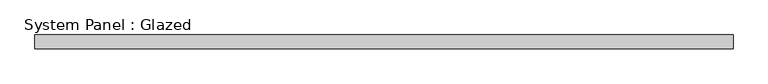
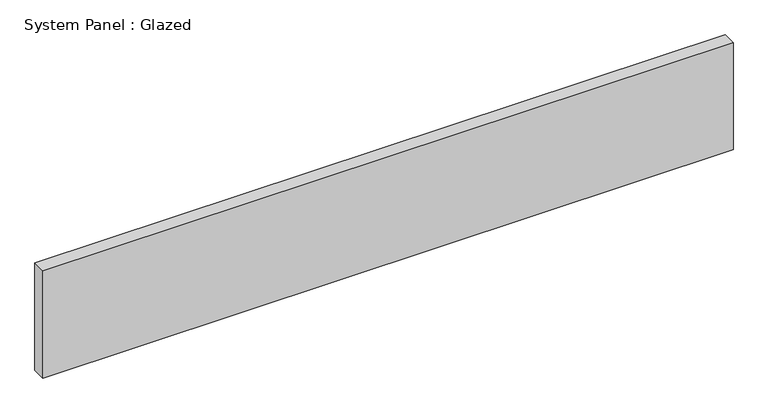
"""IFC4 building model written with IfcOpenShell, lengths in millimetres: plate geometry, System Panel : Glazed."""

from ifc_helpers import new_model, si_unit, origin, origin_with_axes, place, context, project, spatial, polyline, outline, extrude, source, transform, mapped, element, save


def system_panel_glazed_8e393102(model_context):
    return source(origin(), model_context, "Body", "SweptSolid", [
        extrude(outline(polyline([(638.175, 19.05), (-638.175, 19.05), (-638.175, 44.45), (638.175, 44.45), (638.175, 19.05)])), origin_with_axes(), (0.0, 0.0, 1.0), 209.55),
    ])


if __name__ == "__main__":
    model = new_model("IFC4")
    model_context = context("Model", 3, world=origin())
    ifc_project = project(units=[si_unit("LENGTHUNIT", "METRE", prefix="MILLI")], contexts=[model_context])
    site = spatial("IfcSite", under=ifc_project)
    building = spatial("IfcBuilding", under=site)
    placement = place(None, origin())
    system_panel_glazed_shape = system_panel_glazed_8e393102(model_context)
    element("IfcPlate", 1, ObjectType="System Panel : Glazed", at=placement, inside=building, context=model_context, shape_type="MappedRepresentation", body=[
        mapped(system_panel_glazed_shape, transform((0.0, 0.0, 0.0), x_axis=(1.0, 0.0, 0.0), y_axis=(0.0, 1.0, 0.0), z_axis=(0.0, 0.0, 1.0))),
    ])
    save(model, "model.ifc")

# Revit data of these elements
# Type "System Panel : Glazed"
#   Construction Type Id = "GSP4R"
#   Analytic Construction = "1/8 in Pilkington single glazing"
#   Visual Light Transmittance = 0.9
#   Solar Heat Gain Coefficient = 0.86
#   Heat Transfer Coefficient (U) = 1.18115 BTU/(h·ft²·°F)
#   Define Thermal Properties by = 1
# Element 1 (IfcPlate, "System Panel : Glazed")
#   Materials on its faces: "Glass"
# Materials
#   "Glass": class "Glass", colour RGB 0 128 192, transparency 0.75, Description = "Soda Lime Glass", Cost = 0
